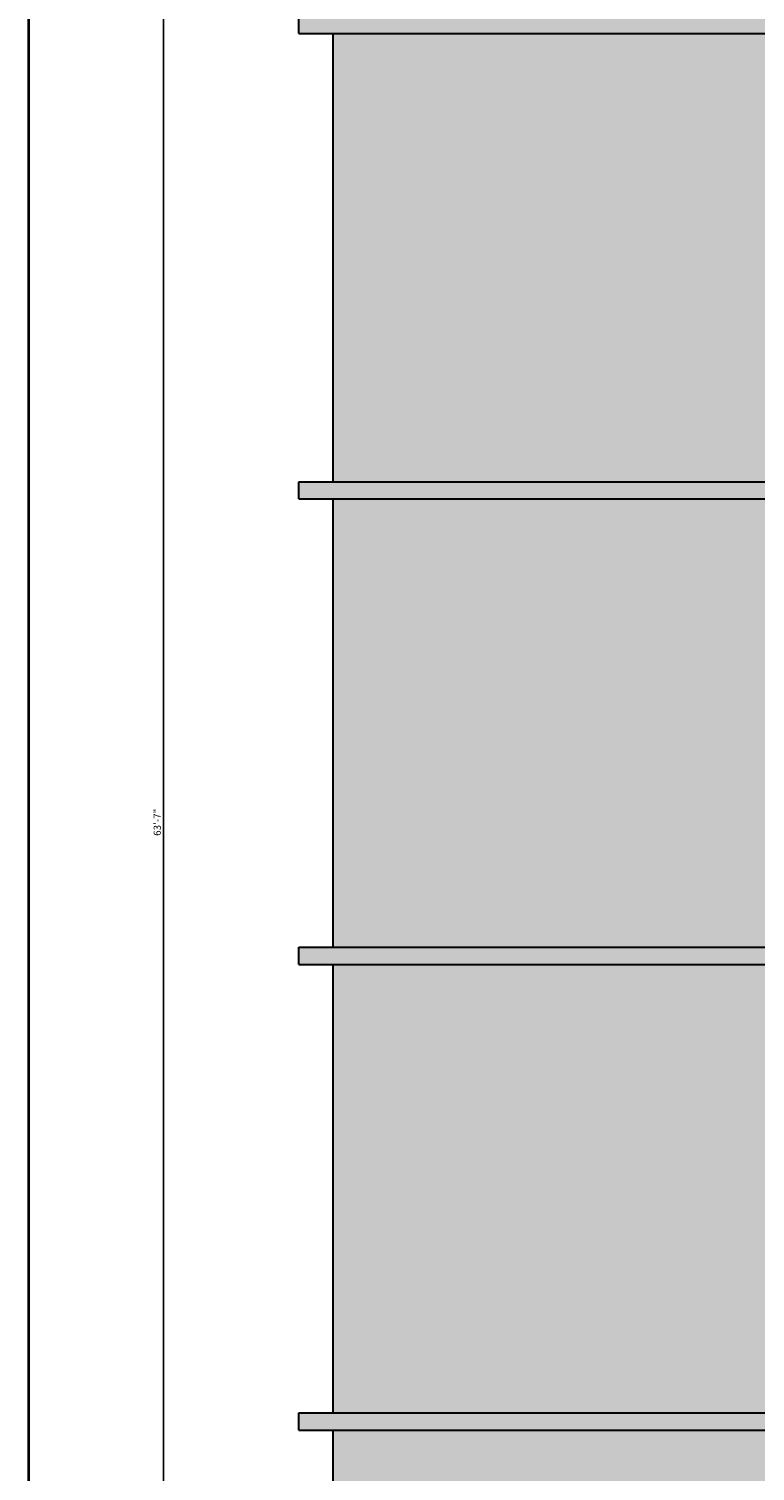
# Model space of a CAD drawing. Units: inches. Extents: x 2391 to 16591, y 7259 to 10239.
# Tile 5 of 27: x 2391 to 2644, y 7745 to 8247. Entities that reach past the tile are written whole.
import ezdxf

# ---------------------------------------------------------------- set-up
doc = ezdxf.new("R2010")
doc.units = ezdxf.units.IN
for name, color, linetype, lineweight in [('A-ANNO-DIMS', 4, 'Continuous', 18), ('A-ANNO-TTLB', 7, 'Continuous', 35), ('A-ELEV', 7, 'Continuous', 30), ('A-ELEV-PATT', 8, 'Continuous', 13), ('A-ELEV-SURF-PATT', 253, 'Continuous', 13)]:
    doc.layers.add(name, color=color, linetype=linetype, lineweight=lineweight)
doc.styles.get("Standard").update_dxf_attribs({"font": 'arial.ttf'})
doc.dimstyles.new('ISO-25', dxfattribs={"dimtxt": 2.5, "dimasz": 2.5, "dimexe": 1.25, "dimexo": 0.625, "dimtad": 1, "dimdec": 0, "dimlunit": 3, "dimtxsty": 'Standard', "dimcen": 2.5, "dimadec": 0, "dimazin": 0, "dimtfac": 1, "dimtdec": 0, "dimtmove": 0, "dimatfit": 3, "dimfxl": 1, "dimarcsym": 0})

# ---------------------------------------------------------------- blocks, each defined once
blk = doc.blocks.new('*D79')
at = {"layer": 'A-ANNO-DIMS', "color": 0, "lineweight": -2, "transparency": 16777216}
for p, q in [((2707.14, 8351.94), (2436.96, 8351.94)), ((2438.21, 7591.44), (2438.21, 8349.44)), ((2490.64, 7588.94), (2436.96, 7588.94))]:
    blk.add_line(p, q, dxfattribs=at)
at = {"layer": 'A-ANNO-DIMS', "color": 0, "transparency": 16777216}
for points in [[(2437.8, 8349.44), (2438.63, 8349.44), (2438.21, 8351.94)], [(2437.8, 7591.44), (2438.63, 7591.44), (2438.21, 7588.94)]]:
    blk.add_solid(points, dxfattribs=at)
at = {"layer": 'Defpoints', "color": 0, "transparency": 16777216}
for p in [(2438.21, 8351.94), (2707.76, 8351.94), (2491.26, 7588.94)]:
    blk.add_point(p, dxfattribs=at)
at = {"layer": 'A-ANNO-DIMS', "color": 0, "transparency": 16777216, "insert": (2436.31, 7970.44), "char_height": 2.5, "attachment_point": 5, "rotation": 90}
blk.add_mtext('63\'-7"', dxfattribs=at)
blk = doc.blocks.new('*D80')
at = {"layer": 'A-ANNO-DIMS', "color": 0, "lineweight": -2, "transparency": 16777216}
for p, q in [((2698.76, 7764.31), (2698.76, 7540.64)), ((2497.26, 7758.31), (2497.26, 7540.64)), ((2499.76, 7541.89), (2696.26, 7541.89))]:
    blk.add_line(p, q, dxfattribs=at)
at = {"layer": 'A-ANNO-DIMS', "color": 0, "transparency": 16777216}
for points in [[(2499.76, 7542.3), (2499.76, 7541.47), (2497.26, 7541.89)], [(2696.26, 7542.3), (2696.26, 7541.47), (2698.76, 7541.89)]]:
    blk.add_solid(points, dxfattribs=at)
at = {"layer": 'Defpoints', "color": 0, "transparency": 16777216}
for p in [(2698.76, 7764.94), (2497.26, 7758.94), (2698.76, 7541.89)]:
    blk.add_point(p, dxfattribs=at)
at = {"layer": 'A-ANNO-DIMS', "color": 0, "transparency": 16777216, "insert": (2598.01, 7543.8), "char_height": 2.5, "attachment_point": 5}
blk.add_mtext('16\'-9 1/2"', dxfattribs=at)

msp = doc.modelspace()

# ---------------------------------------------------------------- hatches: boundary and pattern name
at = {"layer": 'A-ELEV-PATT'}
h = msp.add_hatch(dxfattribs=at)
h.set_pattern_fill('TRIANG', color=256)
h.paths.add_polyline_path([(2698.76, 8244.94), (2497.26, 8244.94), (2497.26, 8088.94), (2698.76, 8088.94)])
h.paths.add_polyline_path([(2649.76, 8172.94), (2649.76, 8190.94), (2679.76, 8190.94), (2679.76, 8172.94)], flags=16)
h.paths.add_polyline_path([(2652.76, 8175.94), (2652.76, 8187.94), (2676.76, 8187.94), (2676.76, 8175.94)], flags=0)
h.paths.add_polyline_path([(2497.26, 8082.94), (2497.26, 7926.94), (2698.76, 7926.94), (2698.76, 8082.94)])
h.paths.add_polyline_path([(2649.76, 8028.94), (2679.76, 8028.94), (2679.76, 8010.94), (2649.76, 8010.94)], flags=16)
h.paths.add_polyline_path([(2652.76, 8025.94), (2676.76, 8025.94), (2676.76, 8013.94), (2652.76, 8013.94)], flags=0)
h.paths.add_polyline_path([(2497.26, 7920.94), (2497.26, 7764.94), (2698.76, 7764.94), (2698.76, 7920.94)])
h.paths.add_polyline_path([(2649.76, 7866.94), (2679.76, 7866.94), (2679.76, 7848.94), (2649.76, 7848.94)], flags=16)
h.paths.add_polyline_path([(2652.76, 7863.94), (2676.76, 7863.94), (2676.76, 7851.94), (2652.76, 7851.94)], flags=0)
at = {"layer": 'A-ELEV-SURF-PATT'}
h = msp.add_hatch(color=256, dxfattribs=at)
h.dxf.hatch_style = 1
h.paths.add_polyline_path([(2941.26, 7764.94), (2485.26, 7764.94), (2485.26, 7758.94), (2941.26, 7758.94)])
h.paths.add_polyline_path([(2941.26, 7920.94), (2941.26, 7926.94), (2485.26, 7926.94), (2485.26, 7920.94)])
h.paths.add_polyline_path([(2941.26, 8082.94), (2941.26, 8088.94), (2485.26, 8088.94), (2485.26, 8082.94)])
h.paths.add_polyline_path([(2485.26, 8250.94), (2485.26, 8244.94), (2941.26, 8244.94), (2941.26, 8250.94)])
h.paths.add_polyline_path([(2707.76, 8351.94), (2707.76, 8346.94), (2908.26, 8346.94), (2908.26, 8351.94)])
h = msp.add_hatch(color=256, dxfattribs=at)
h.dxf.hatch_style = 1
h.paths.add_polyline_path([(2929.26, 7758.94), (2497.26, 7758.94), (2497.26, 7715.94), (2690.26, 7715.94), (2690.26, 7724.94), (2685.26, 7724.94), (2685.26, 7729.94), (2704.26, 7729.94), (2704.26, 7724.94), (2699.26, 7724.94), (2699.26, 7695.78), (2701.76, 7695.78), (2701.76, 7697.78), (2704.26, 7697.78), (2704.26, 7722.94), (2773.26, 7722.94), (2773.26, 7607.94), (2704.26, 7607.94), (2704.26, 7602.94), (2843.26, 7602.94), (2843.26, 7607.94), (2774.26, 7607.94), (2774.26, 7722.94), (2843.26, 7722.94), (2843.26, 7697.78), (2845.76, 7697.78), (2845.76, 7695.78), (2848.26, 7695.78), (2848.26, 7724.94), (2843.26, 7724.94), (2843.26, 7729.94), (2862.26, 7729.94), (2862.26, 7724.94), (2857.26, 7724.94), (2857.26, 7715.94), (2929.26, 7715.94)])
h.paths.add_polyline_path([(2848.26, 7693.78), (2845.76, 7693.78), (2845.76, 7691.78), (2843.26, 7691.78), (2843.26, 7637.65), (2845.76, 7637.65), (2845.76, 7635.65), (2848.26, 7635.65)], flags=17)
h.paths.add_polyline_path([(2848.26, 7633.65), (2845.76, 7633.65), (2845.76, 7631.65), (2843.26, 7631.65), (2843.26, 7602.94), (2848.26, 7602.94)], flags=17)
h.paths.add_polyline_path([(2704.26, 7631.65), (2701.76, 7631.65), (2701.76, 7633.65), (2699.26, 7633.65), (2699.26, 7602.94), (2704.26, 7602.94), (2704.26, 7607.94)], flags=17)
h.paths.add_polyline_path([(2704.26, 7691.78), (2701.76, 7691.78), (2701.76, 7693.78), (2699.26, 7693.78), (2699.26, 7635.65), (2701.76, 7635.65), (2701.76, 7637.65), (2704.26, 7637.65)], flags=17)

# ---------------------------------------------------------------- linework, layer by layer
at = {"layer": 'A-ANNO-TTLB'}
msp.add_lwpolyline([(2391.28, 10239.38), (4154.2, 10239.38), (4154.2, 7258.54), (2391.28, 7258.54)], close=True, dxfattribs=at)
at = {"layer": 'A-ELEV'}
for p, q in [((2485.26, 8244.94), (2485.26, 8250.94)), ((2485.26, 8244.94), (2941.26, 8244.94)), ((2497.26, 8088.94), (2497.26, 8244.94)), ((2485.26, 8088.94), (2941.26, 8088.94)), ((2485.26, 8082.94), (2485.26, 8088.94)), ((2485.26, 8082.94), (2941.26, 8082.94)), ((2497.26, 7926.94), (2497.26, 8082.94)), ((2485.26, 7926.94), (2941.26, 7926.94)), ((2485.26, 7920.94), (2485.26, 7926.94)), ((2485.26, 7920.94), (2941.26, 7920.94)), ((2497.26, 7764.94), (2497.26, 7920.94)), ((2485.26, 7764.94), (2941.26, 7764.94)), ((2485.26, 7758.94), (2485.26, 7764.94)), ((2485.26, 7758.94), (2941.26, 7758.94)), ((2497.26, 7593.94), (2497.26, 7758.94))]:
    msp.add_line(p, q, dxfattribs=at)

# ---------------------------------------------------------------- dimensions: what is measured, and where the dimension line sits
at = {"layer": 'A-ANNO-DIMS'}
dim = msp.add_linear_dim(base=(2438.21, 8351.94), p1=(2491.26, 7588.94), p2=(2707.76, 8351.94), angle=90, dimstyle='ISO-25', override={"dimdec": 1, "dimlfac": 1, "dimrnd": 0, "dimzin": 1, "dimdsep": 46, "dimlunit": 4, "dimfrac": 2}, dxfattribs=at)
dim.commit()
dim.dimension.update_dxf_attribs({"geometry": '*D79', "text_midpoint": (2436.31, 7970.44)})
dim = msp.add_linear_dim(base=(2698.76, 7541.89), p1=(2497.26, 7758.94), p2=(2698.76, 7764.94), dimstyle='ISO-25', override={"dimdec": 1, "dimlfac": 1, "dimrnd": 0, "dimzin": 1, "dimdsep": 46, "dimlunit": 4, "dimfrac": 2}, dxfattribs=at)
dim.commit()
dim.dimension.update_dxf_attribs({"geometry": '*D80', "text_midpoint": (2598.01, 7543.8)})

doc.saveas('drawing.dxf')
